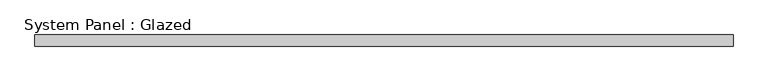
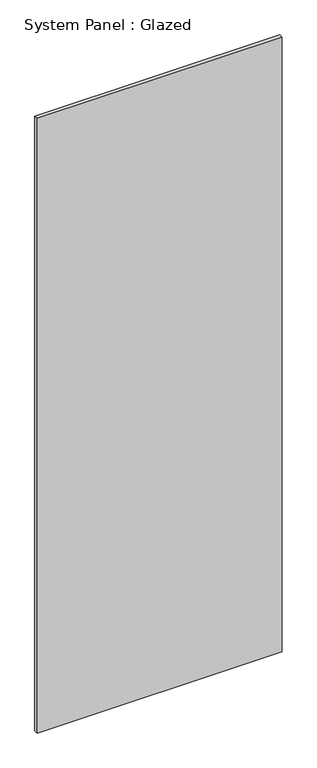
"""IFC4 building model written with IfcOpenShell, lengths in millimetres: plate geometry, System Panel : Glazed."""

from ifc_helpers import new_model, si_unit, origin, origin_with_axes, place, context, project, spatial, polyline, outline, extrude, source, transform, mapped, element, save


def system_panel_glazed_61de1ab3(model_context):
    return source(origin(), model_context, "Body", "SweptSolid", [
        extrude(outline(polyline([(754.4921342, 24.5), (-754.4921342, 24.5), (-754.4921342, 49.5), (754.4921342, 49.5), (754.4921342, 24.5)])), origin_with_axes(), (0.0, 0.0, 1.0), 4000.0),
    ])


if __name__ == "__main__":
    model = new_model("IFC4")
    model_context = context("Model", 3, world=origin())
    ifc_project = project(units=[si_unit("LENGTHUNIT", "METRE", prefix="MILLI")], contexts=[model_context])
    site = spatial("IfcSite", under=ifc_project)
    building = spatial("IfcBuilding", under=site)
    placement = place(None, origin())
    system_panel_glazed_shape = system_panel_glazed_61de1ab3(model_context)
    element("IfcPlate", 1, ObjectType="System Panel : Glazed", at=placement, inside=building, context=model_context, shape_type="MappedRepresentation", body=[
        mapped(system_panel_glazed_shape, transform((0.0, 0.0, 0.0), x_axis=(1.0, 0.0, 0.0), y_axis=(0.0, 1.0, 0.0), z_axis=(0.0, 0.0, 1.0))),
    ])
    save(model, "model.ifc")

# Revit data of these elements
# Type "System Panel : Glazed"
#   Keynote = "H11"
#   Construction Type Id = "GSP4R"
#   Analytic Construction = "1/8 in Pilkington single glazing"
#   Visual Light Transmittance = 0.9
#   Solar Heat Gain Coefficient = 0.86
#   Heat Transfer Coefficient (U) = 6.7069 W/(m²·K)
#   Define Thermal Properties by = 1
# Element 1 (IfcPlate, "System Panel : Glazed")
#   Materials on its faces: "Glass"
# Materials
#   "Glass": class "Glass", colour RGB 0 128 192, transparency 0.9, Description = "Soda Lime Glass", Cost = 0
